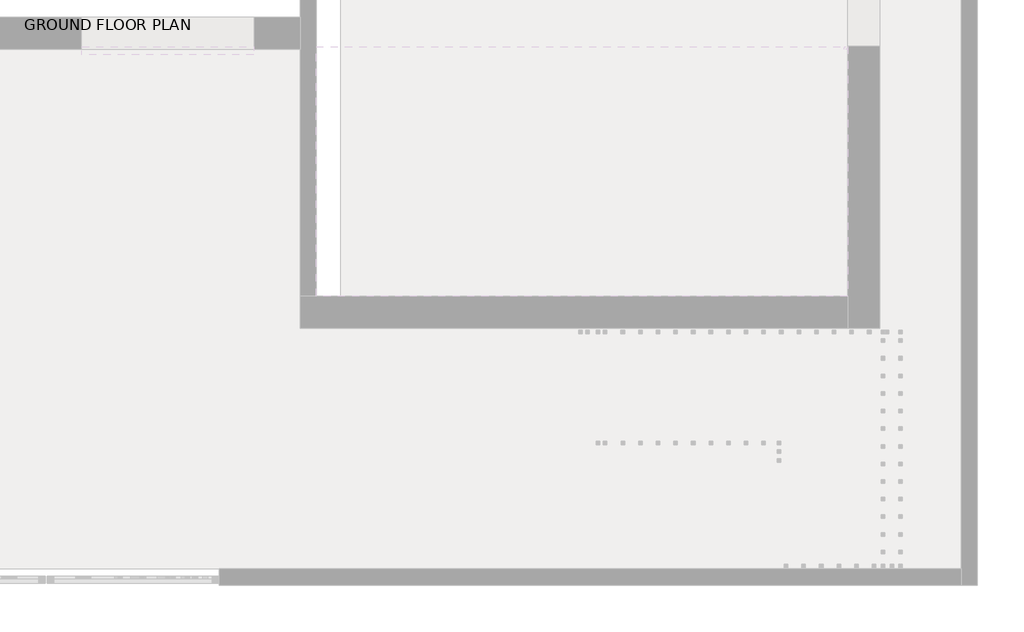
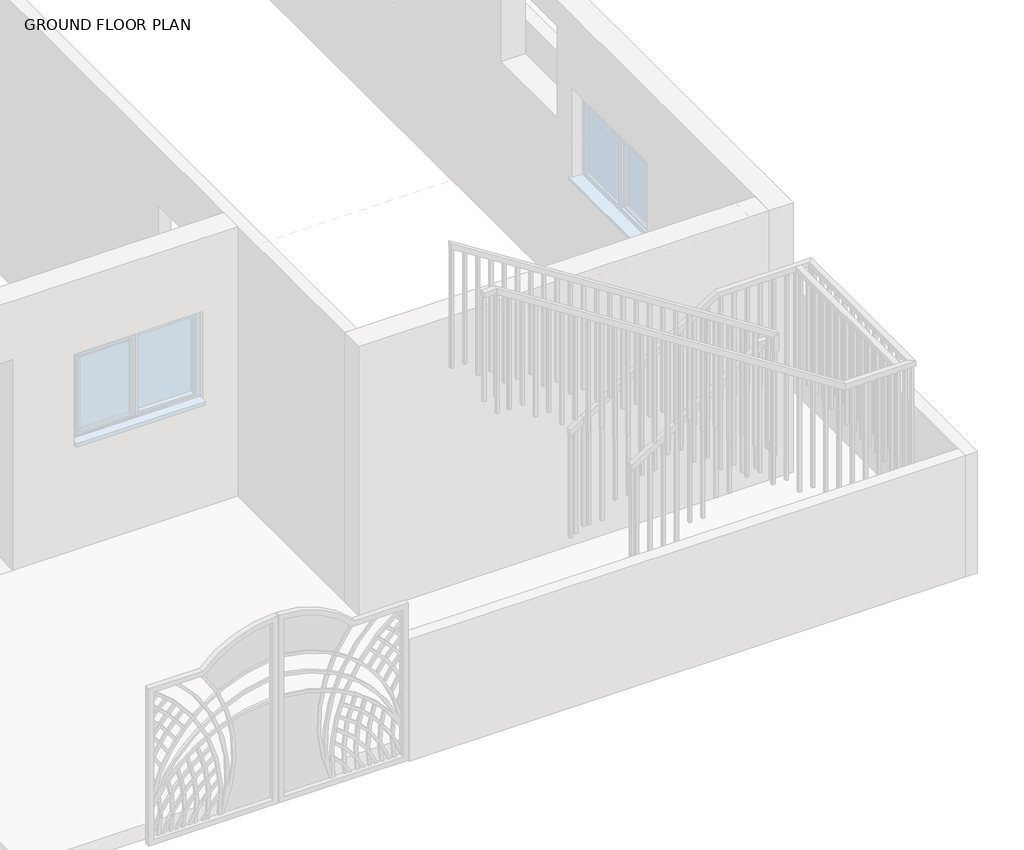
# One storey, part 22 of 23: 2 railings.
"""IFC4 building model written with IfcOpenShell, lengths in millimetres."""

from ifc_helpers import new_model, si_unit, frame, origin, place, context, project, spatial, polyline, outline, extrude, faceted_brep, element, save

model = new_model("IFC4")

# Units and contexts
model_context = context("Model", 3, world=origin())
ifc_project = project(units=[si_unit("LENGTHUNIT", "METRE", prefix="MILLI")], contexts=[model_context])

# Site, building, storey
site = spatial("IfcSite", under=ifc_project)
building = spatial("IfcBuilding", under=site)
storey = spatial("IfcBuildingStorey", under=building, Name="GROUND FLOOR PLAN", Elevation=487.68)

# Railings
placement = place(None, origin())
element("IfcRailing", 1, ObjectType="1100mm", at=placement, inside=storey, context=model_context, shape_type="SolidModel", body=[
    faceted_brep([(-8680.149573, -10220.0521308, 1912.8), (-8680.149573, -10220.0521308, 1853.4423995), (-8680.149573, -10270.0521308, 1853.4423995), (-8680.149573, -10270.0521308, 1912.8), (-7409.7306254, -10220.0521308, 2725.6), (-7395.1045513, -10220.0521308, 2675.6), (-7395.1045513, -10270.0521308, 2675.6), (-7409.7306254, -10270.0521308, 2725.6), (-6495.8132565, -10220.0521308, 2725.6), (-6495.8132565, -10220.0521308, 2675.6), (-6545.8132565, -10270.0521308, 2675.6), (-6545.8132565, -10270.0521308, 2725.6), (-6495.8132565, -11933.6860066, 2725.6), (-6495.8132565, -11933.6860066, 2675.6), (-6545.8132565, -11883.6860066, 2675.6), (-6545.8132565, -11883.6860066, 2725.6), (-7155.718398, -11933.6860066, 2725.6), (-7170.3479429, -11933.6860066, 2675.6), (-7170.3479429, -11883.6860066, 2675.6), (-7155.718398, -11883.6860066, 2725.6), (-10457.8773536, -11933.6860066, 4838.88), (-10457.8773536, -11883.6860066, 4838.88), (-10457.8773536, -11883.6860066, 4779.517542), (-10457.8773536, -11933.6860066, 4779.517542)], [[[0, 1, 2, 3]], [[1, 0, 4, 5]], [[2, 1, 5, 6]], [[3, 2, 6, 7]], [[0, 3, 7, 4]], [[5, 4, 8, 9]], [[6, 5, 9, 10]], [[7, 6, 10, 11]], [[4, 7, 11, 8]], [[9, 8, 12, 13]], [[10, 9, 13, 14]], [[11, 10, 14, 15]], [[8, 11, 15, 12]], [[13, 12, 16, 17]], [[14, 13, 17, 18]], [[15, 14, 18, 19]], [[12, 15, 19, 16]], [[20, 21, 22, 23]], [[17, 16, 20, 23]], [[18, 17, 23, 22]], [[19, 18, 22, 21]], [[16, 19, 21, 20]]]),
    extrude(outline(polyline([(4691.8007425, -10320.8132565), (4707.7999723, -10345.8132565), (3576.32, -10345.8132565), (3576.32, -10320.8132565), (4691.8007425, -10320.8132565)])), frame((0.0, -11921.1860066, 0.0), z_axis=(0.0, 1.0, 0.0), x_axis=(0.0, 0.0, 1.0)), (0.0, 0.0, 1.0), 25.0),
    extrude(outline(polyline([(4611.8045935, -10195.8132565), (4627.8038233, -10220.8132565), (3576.32, -10220.8132565), (3576.32, -10195.8132565), (4611.8045935, -10195.8132565)])), frame((0.0, -11921.1860066, 0.0), z_axis=(0.0, 1.0, 0.0), x_axis=(0.0, 0.0, 1.0)), (0.0, 0.0, 1.0), 25.0),
    extrude(outline(polyline([(4531.8084444, -10070.8132565), (4547.8076742, -10095.8132565), (3413.76, -10095.8132565), (3413.76, -10070.8132565), (4531.8084444, -10070.8132565)])), frame((0.0, -11921.1860066, 0.0), z_axis=(0.0, 1.0, 0.0), x_axis=(0.0, 0.0, 1.0)), (0.0, 0.0, 1.0), 25.0),
    extrude(outline(polyline([(4451.8122954, -9945.8132565), (4467.8115252, -9970.8132565), (3413.76, -9970.8132565), (3413.76, -9945.8132565), (4451.8122954, -9945.8132565)])), frame((0.0, -11921.1860066, 0.0), z_axis=(0.0, 1.0, 0.0), x_axis=(0.0, 0.0, 1.0)), (0.0, 0.0, 1.0), 25.0),
    extrude(outline(polyline([(4371.8161463, -9820.8132565), (4387.8153761, -9845.8132565), (3251.2, -9845.8132565), (3251.2, -9820.8132565), (4371.8161463, -9820.8132565)])), frame((0.0, -11921.1860066, 0.0), z_axis=(0.0, 1.0, 0.0), x_axis=(0.0, 0.0, 1.0)), (0.0, 0.0, 1.0), 25.0),
    extrude(outline(polyline([(4291.8423995, -9695.8132565), (4307.8371231, -9720.8132565), (3251.2, -9720.8132565), (3251.2, -9695.8132565), (4291.8423995, -9695.8132565)])), frame((0.0, -11921.1860066, 0.0), z_axis=(0.0, 1.0, 0.0), x_axis=(0.0, 0.0, 1.0)), (0.0, 0.0, 1.0), 25.0),
    extrude(outline(polyline([(4211.8238482, -9570.8132565), (4227.823078, -9595.8132565), (3088.64, -9595.8132565), (3088.64, -9570.8132565), (4211.8238482, -9570.8132565)])), frame((0.0, -11921.1860066, 0.0), z_axis=(0.0, 1.0, 0.0), x_axis=(0.0, 0.0, 1.0)), (0.0, 0.0, 1.0), 25.0),
    extrude(outline(polyline([(4131.8276992, -9445.8132565), (4147.826929, -9470.8132565), (3088.64, -9470.8132565), (3088.64, -9445.8132565), (4131.8276992, -9445.8132565)])), frame((0.0, -11921.1860066, 0.0), z_axis=(0.0, 1.0, 0.0), x_axis=(0.0, 0.0, 1.0)), (0.0, 0.0, 1.0), 25.0),
    extrude(outline(polyline([(4051.8315501, -9320.8132565), (4067.8307799, -9345.8132565), (2926.08, -9345.8132565), (2926.08, -9320.8132565), (4051.8315501, -9320.8132565)])), frame((0.0, -11921.1860066, 0.0), z_axis=(0.0, 1.0, 0.0), x_axis=(0.0, 0.0, 1.0)), (0.0, 0.0, 1.0), 25.0),
    extrude(outline(polyline([(3971.835401, -9195.8132565), (3987.8346309, -9220.8132565), (2926.08, -9220.8132565), (2926.08, -9195.8132565), (3971.835401, -9195.8132565)])), frame((0.0, -11921.1860066, 0.0), z_axis=(0.0, 1.0, 0.0), x_axis=(0.0, 0.0, 1.0)), (0.0, 0.0, 1.0), 25.0),
    extrude(outline(polyline([(3891.839252, -9070.8132565), (3907.8384818, -9095.8132565), (2763.52, -9095.8132565), (2763.52, -9070.8132565), (3891.839252, -9070.8132565)])), frame((0.0, -11921.1860066, 0.0), z_axis=(0.0, 1.0, 0.0), x_axis=(0.0, 0.0, 1.0)), (0.0, 0.0, 1.0), 25.0),
    extrude(outline(polyline([(3811.8431029, -8945.8132565), (3827.8423328, -8970.8132565), (2763.52, -8970.8132565), (2763.52, -8945.8132565), (3811.8431029, -8945.8132565)])), frame((0.0, -11921.1860066, 0.0), z_axis=(0.0, 1.0, 0.0), x_axis=(0.0, 0.0, 1.0)), (0.0, 0.0, 1.0), 25.0),
    extrude(outline(polyline([(3731.8469539, -8820.8132565), (3747.8461837, -8845.8132565), (2600.96, -8845.8132565), (2600.96, -8820.8132565), (3731.8469539, -8820.8132565)])), frame((0.0, -11921.1860066, 0.0), z_axis=(0.0, 1.0, 0.0), x_axis=(0.0, 0.0, 1.0)), (0.0, 0.0, 1.0), 25.0),
    extrude(outline(polyline([(3651.8508048, -8695.8132565), (3667.8500347, -8720.8132565), (2600.96, -8720.8132565), (2600.96, -8695.8132565), (3651.8508048, -8695.8132565)])), frame((0.0, -11921.1860066, 0.0), z_axis=(0.0, 1.0, 0.0), x_axis=(0.0, 0.0, 1.0)), (0.0, 0.0, 1.0), 25.0),
    extrude(outline(polyline([(3571.8546558, -8570.8132565), (3587.8538856, -8595.8132565), (2438.4, -8595.8132565), (2438.4, -8570.8132565), (3571.8546558, -8570.8132565)])), frame((0.0, -11921.1860066, 0.0), z_axis=(0.0, 1.0, 0.0), x_axis=(0.0, 0.0, 1.0)), (0.0, 0.0, 1.0), 25.0),
    extrude(outline(polyline([(3491.8585067, -8445.8132565), (3507.8577365, -8470.8132565), (2438.4, -8470.8132565), (2438.4, -8445.8132565), (3491.8585067, -8445.8132565)])), frame((0.0, -11921.1860066, 0.0), z_axis=(0.0, 1.0, 0.0), x_axis=(0.0, 0.0, 1.0)), (0.0, 0.0, 1.0), 25.0),
    extrude(outline(polyline([(3411.8623577, -8320.8132565), (3427.8615875, -8345.8132565), (2275.84, -8345.8132565), (2275.84, -8320.8132565), (3411.8623577, -8320.8132565)])), frame((0.0, -11921.1860066, 0.0), z_axis=(0.0, 1.0, 0.0), x_axis=(0.0, 0.0, 1.0)), (0.0, 0.0, 1.0), 25.0),
    extrude(outline(polyline([(3331.8662086, -8195.8132565), (3347.8654384, -8220.8132565), (2275.84, -8220.8132565), (2275.84, -8195.8132565), (3331.8662086, -8195.8132565)])), frame((0.0, -11921.1860066, 0.0), z_axis=(0.0, 1.0, 0.0), x_axis=(0.0, 0.0, 1.0)), (0.0, 0.0, 1.0), 25.0),
    extrude(outline(polyline([(3251.8700596, -8070.8132565), (3267.8692894, -8095.8132565), (2113.28, -8095.8132565), (2113.28, -8070.8132565), (3251.8700596, -8070.8132565)])), frame((0.0, -11921.1860066, 0.0), z_axis=(0.0, 1.0, 0.0), x_axis=(0.0, 0.0, 1.0)), (0.0, 0.0, 1.0), 25.0),
    extrude(outline(polyline([(3171.8739105, -7945.8132565), (3187.8731403, -7970.8132565), (2113.28, -7970.8132565), (2113.28, -7945.8132565), (3171.8739105, -7945.8132565)])), frame((0.0, -11921.1860066, 0.0), z_axis=(0.0, 1.0, 0.0), x_axis=(0.0, 0.0, 1.0)), (0.0, 0.0, 1.0), 25.0),
    extrude(outline(polyline([(3091.8777615, -7820.8132565), (3107.8769913, -7845.8132565), (1950.72, -7845.8132565), (1950.72, -7820.8132565), (3091.8777615, -7820.8132565)])), frame((0.0, -11921.1860066, 0.0), z_axis=(0.0, 1.0, 0.0), x_axis=(0.0, 0.0, 1.0)), (0.0, 0.0, 1.0), 25.0),
    extrude(outline(polyline([(3011.8816124, -7695.8132565), (3027.8808422, -7720.8132565), (1950.72, -7720.8132565), (1950.72, -7695.8132565), (3011.8816124, -7695.8132565)])), frame((0.0, -11921.1860066, 0.0), z_axis=(0.0, 1.0, 0.0), x_axis=(0.0, 0.0, 1.0)), (0.0, 0.0, 1.0), 25.0),
    extrude(outline(polyline([(2931.8854634, -7570.8132565), (2947.8846932, -7595.8132565), (1788.16, -7595.8132565), (1788.16, -7570.8132565), (2931.8854634, -7570.8132565)])), frame((0.0, -11921.1860066, 0.0), z_axis=(0.0, 1.0, 0.0), x_axis=(0.0, 0.0, 1.0)), (0.0, 0.0, 1.0), 25.0),
    extrude(outline(polyline([(2851.8893143, -7445.8132565), (2867.8885441, -7470.8132565), (1788.16, -7470.8132565), (1788.16, -7445.8132565), (2851.8893143, -7445.8132565)])), frame((0.0, -11921.1860066, 0.0), z_axis=(0.0, 1.0, 0.0), x_axis=(0.0, 0.0, 1.0)), (0.0, 0.0, 1.0), 25.0),
    extrude(outline(polyline([(2771.8931653, -7320.8132565), (2787.8923951, -7345.8132565), (1625.6, -7345.8132565), (1625.6, -7320.8132565), (2771.8931653, -7320.8132565)])), frame((0.0, -11921.1860066, 0.0), z_axis=(0.0, 1.0, 0.0), x_axis=(0.0, 0.0, 1.0)), (0.0, 0.0, 1.0), 25.0),
    extrude(outline(polyline([(2691.8970162, -7195.8132565), (2707.896246, -7220.8132565), (1625.6, -7220.8132565), (1625.6, -7195.8132565), (2691.8970162, -7195.8132565)])), frame((0.0, -11921.1860066, 0.0), z_axis=(0.0, 1.0, 0.0), x_axis=(0.0, 0.0, 1.0)), (0.0, 0.0, 1.0), 25.0),
    extrude(outline(polyline([(-7070.8132565, -11921.1860066), (-7095.8132565, -11921.1860066), (-7095.8132565, -11896.1860066), (-7070.8132565, -11896.1860066), (-7070.8132565, -11921.1860066)])), frame((0.0, 0.0, 1625.6), z_axis=(0.0, 0.0, 1.0), x_axis=(1.0, 0.0, 0.0)), (0.0, 0.0, 1.0), 1050.0),
    extrude(outline(polyline([(-6945.8132565, -11921.1860066), (-6970.8132565, -11921.1860066), (-6970.8132565, -11896.1860066), (-6945.8132565, -11896.1860066), (-6945.8132565, -11921.1860066)])), frame((0.0, 0.0, 1625.6), z_axis=(0.0, 0.0, 1.0), x_axis=(1.0, 0.0, 0.0)), (0.0, 0.0, 1.0), 1050.0),
    extrude(outline(polyline([(-6820.8132565, -11921.1860066), (-6845.8132565, -11921.1860066), (-6845.8132565, -11896.1860066), (-6820.8132565, -11896.1860066), (-6820.8132565, -11921.1860066)])), frame((0.0, 0.0, 1625.6), z_axis=(0.0, 0.0, 1.0), x_axis=(1.0, 0.0, 0.0)), (0.0, 0.0, 1.0), 1050.0),
    extrude(outline(polyline([(-6695.8132565, -11921.1860066), (-6720.8132565, -11921.1860066), (-6720.8132565, -11896.1860066), (-6695.8132565, -11896.1860066), (-6695.8132565, -11921.1860066)])), frame((0.0, 0.0, 1625.6), z_axis=(0.0, 0.0, 1.0), x_axis=(1.0, 0.0, 0.0)), (0.0, 0.0, 1.0), 1050.0),
    extrude(outline(polyline([(-6570.8132565, -11921.1860066), (-6595.8132565, -11921.1860066), (-6595.8132565, -11896.1860066), (-6570.8132565, -11896.1860066), (-6570.8132565, -11921.1860066)])), frame((0.0, 0.0, 1625.6), z_axis=(0.0, 0.0, 1.0), x_axis=(1.0, 0.0, 0.0)), (0.0, 0.0, 1.0), 1050.0),
    extrude(outline(polyline([(-6508.3132565, -11795.0521308), (-6508.3132565, -11820.0521308), (-6533.3132565, -11820.0521308), (-6533.3132565, -11795.0521308), (-6508.3132565, -11795.0521308)])), frame((0.0, 0.0, 1625.6), z_axis=(0.0, 0.0, 1.0), x_axis=(1.0, 0.0, 0.0)), (0.0, 0.0, 1.0), 1050.0),
    extrude(outline(polyline([(-6508.3132565, -11670.0521308), (-6508.3132565, -11695.0521308), (-6533.3132565, -11695.0521308), (-6533.3132565, -11670.0521308), (-6508.3132565, -11670.0521308)])), frame((0.0, 0.0, 1625.6), z_axis=(0.0, 0.0, 1.0), x_axis=(1.0, 0.0, 0.0)), (0.0, 0.0, 1.0), 1050.0),
    extrude(outline(polyline([(-6508.3132565, -11545.0521308), (-6508.3132565, -11570.0521308), (-6533.3132565, -11570.0521308), (-6533.3132565, -11545.0521308), (-6508.3132565, -11545.0521308)])), frame((0.0, 0.0, 1625.6), z_axis=(0.0, 0.0, 1.0), x_axis=(1.0, 0.0, 0.0)), (0.0, 0.0, 1.0), 1050.0),
    extrude(outline(polyline([(-6508.3132565, -11420.0521308), (-6508.3132565, -11445.0521308), (-6533.3132565, -11445.0521308), (-6533.3132565, -11420.0521308), (-6508.3132565, -11420.0521308)])), frame((0.0, 0.0, 1625.6), z_axis=(0.0, 0.0, 1.0), x_axis=(1.0, 0.0, 0.0)), (0.0, 0.0, 1.0), 1050.0),
    extrude(outline(polyline([(-6508.3132565, -11295.0521308), (-6508.3132565, -11320.0521308), (-6533.3132565, -11320.0521308), (-6533.3132565, -11295.0521308), (-6508.3132565, -11295.0521308)])), frame((0.0, 0.0, 1625.6), z_axis=(0.0, 0.0, 1.0), x_axis=(1.0, 0.0, 0.0)), (0.0, 0.0, 1.0), 1050.0),
    extrude(outline(polyline([(-6508.3132565, -11170.0521308), (-6508.3132565, -11195.0521308), (-6533.3132565, -11195.0521308), (-6533.3132565, -11170.0521308), (-6508.3132565, -11170.0521308)])), frame((0.0, 0.0, 1625.6), z_axis=(0.0, 0.0, 1.0), x_axis=(1.0, 0.0, 0.0)), (0.0, 0.0, 1.0), 1050.0),
    extrude(outline(polyline([(-6508.3132565, -11045.0521308), (-6508.3132565, -11070.0521308), (-6533.3132565, -11070.0521308), (-6533.3132565, -11045.0521308), (-6508.3132565, -11045.0521308)])), frame((0.0, 0.0, 1625.6), z_axis=(0.0, 0.0, 1.0), x_axis=(1.0, 0.0, 0.0)), (0.0, 0.0, 1.0), 1050.0),
    extrude(outline(polyline([(-6508.3132565, -10920.0521308), (-6508.3132565, -10945.0521308), (-6533.3132565, -10945.0521308), (-6533.3132565, -10920.0521308), (-6508.3132565, -10920.0521308)])), frame((0.0, 0.0, 1625.6), z_axis=(0.0, 0.0, 1.0), x_axis=(1.0, 0.0, 0.0)), (0.0, 0.0, 1.0), 1050.0),
    extrude(outline(polyline([(-6508.3132565, -10795.0521308), (-6508.3132565, -10820.0521308), (-6533.3132565, -10820.0521308), (-6533.3132565, -10795.0521308), (-6508.3132565, -10795.0521308)])), frame((0.0, 0.0, 1625.6), z_axis=(0.0, 0.0, 1.0), x_axis=(1.0, 0.0, 0.0)), (0.0, 0.0, 1.0), 1050.0),
    extrude(outline(polyline([(-6508.3132565, -10670.0521308), (-6508.3132565, -10695.0521308), (-6533.3132565, -10695.0521308), (-6533.3132565, -10670.0521308), (-6508.3132565, -10670.0521308)])), frame((0.0, 0.0, 1625.6), z_axis=(0.0, 0.0, 1.0), x_axis=(1.0, 0.0, 0.0)), (0.0, 0.0, 1.0), 1050.0),
    extrude(outline(polyline([(-6508.3132565, -10545.0521308), (-6508.3132565, -10570.0521308), (-6533.3132565, -10570.0521308), (-6533.3132565, -10545.0521308), (-6508.3132565, -10545.0521308)])), frame((0.0, 0.0, 1625.6), z_axis=(0.0, 0.0, 1.0), x_axis=(1.0, 0.0, 0.0)), (0.0, 0.0, 1.0), 1050.0),
    extrude(outline(polyline([(-6508.3132565, -10420.0521308), (-6508.3132565, -10445.0521308), (-6533.3132565, -10445.0521308), (-6533.3132565, -10420.0521308), (-6508.3132565, -10420.0521308)])), frame((0.0, 0.0, 1625.6), z_axis=(0.0, 0.0, 1.0), x_axis=(1.0, 0.0, 0.0)), (0.0, 0.0, 1.0), 1050.0),
    extrude(outline(polyline([(-6508.3132565, -10295.0521308), (-6508.3132565, -10320.0521308), (-6533.3132565, -10320.0521308), (-6533.3132565, -10295.0521308), (-6508.3132565, -10295.0521308)])), frame((0.0, 0.0, 1625.6), z_axis=(0.0, 0.0, 1.0), x_axis=(1.0, 0.0, 0.0)), (0.0, 0.0, 1.0), 1050.0),
    extrude(outline(polyline([(-6630.149573, -10232.5521308), (-6605.149573, -10232.5521308), (-6605.149573, -10257.5521308), (-6630.149573, -10257.5521308), (-6630.149573, -10232.5521308)])), frame((0.0, 0.0, 1625.6), z_axis=(0.0, 0.0, 1.0), x_axis=(1.0, 0.0, 0.0)), (0.0, 0.0, 1.0), 1050.0),
    extrude(outline(polyline([(-6755.149573, -10232.5521308), (-6730.149573, -10232.5521308), (-6730.149573, -10257.5521308), (-6755.149573, -10257.5521308), (-6755.149573, -10232.5521308)])), frame((0.0, 0.0, 1625.6), z_axis=(0.0, 0.0, 1.0), x_axis=(1.0, 0.0, 0.0)), (0.0, 0.0, 1.0), 1050.0),
    extrude(outline(polyline([(-6880.149573, -10232.5521308), (-6855.149573, -10232.5521308), (-6855.149573, -10257.5521308), (-6880.149573, -10257.5521308), (-6880.149573, -10232.5521308)])), frame((0.0, 0.0, 1625.6), z_axis=(0.0, 0.0, 1.0), x_axis=(1.0, 0.0, 0.0)), (0.0, 0.0, 1.0), 1050.0),
    extrude(outline(polyline([(-7005.149573, -10232.5521308), (-6980.149573, -10232.5521308), (-6980.149573, -10257.5521308), (-7005.149573, -10257.5521308), (-7005.149573, -10232.5521308)])), frame((0.0, 0.0, 1625.6), z_axis=(0.0, 0.0, 1.0), x_axis=(1.0, 0.0, 0.0)), (0.0, 0.0, 1.0), 1050.0),
    extrude(outline(polyline([(-7130.149573, -10232.5521308), (-7105.149573, -10232.5521308), (-7105.149573, -10257.5521308), (-7130.149573, -10257.5521308), (-7130.149573, -10232.5521308)])), frame((0.0, 0.0, 1625.6), z_axis=(0.0, 0.0, 1.0), x_axis=(1.0, 0.0, 0.0)), (0.0, 0.0, 1.0), 1050.0),
    extrude(outline(polyline([(-7255.149573, -10232.5521308), (-7230.149573, -10232.5521308), (-7230.149573, -10257.5521308), (-7255.149573, -10257.5521308), (-7255.149573, -10232.5521308)])), frame((0.0, 0.0, 1625.6), z_axis=(0.0, 0.0, 1.0), x_axis=(1.0, 0.0, 0.0)), (0.0, 0.0, 1.0), 1050.0),
    extrude(outline(polyline([(-7380.149573, -10232.5521308), (-7355.149573, -10232.5521308), (-7355.149573, -10257.5521308), (-7380.149573, -10257.5521308), (-7380.149573, -10232.5521308)])), frame((0.0, 0.0, 1625.6), z_axis=(0.0, 0.0, 1.0), x_axis=(1.0, 0.0, 0.0)), (0.0, 0.0, 1.0), 1050.0),
    extrude(outline(polyline([(1463.04, -7505.149573), (1463.04, -7480.149573), (2621.1891352, -7480.149573), (2605.1944115, -7505.149573), (1463.04, -7505.149573)])), frame((0.0, -10257.5521308, 0.0), z_axis=(0.0, 1.0, 0.0), x_axis=(0.0, 0.0, 1.0)), (0.0, 0.0, 1.0), 25.0),
    extrude(outline(polyline([(1463.04, -7630.149573), (1463.04, -7605.149573), (2541.2155169, -7605.149573), (2525.2207932, -7630.149573), (1463.04, -7630.149573)])), frame((0.0, -10257.5521308, 0.0), z_axis=(0.0, 1.0, 0.0), x_axis=(0.0, 0.0, 1.0)), (0.0, 0.0, 1.0), 25.0),
    extrude(outline(polyline([(1300.48, -7755.149573), (1300.48, -7730.149573), (2461.2418986, -7730.149573), (2445.2471749, -7755.149573), (1300.48, -7755.149573)])), frame((0.0, -10257.5521308, 0.0), z_axis=(0.0, 1.0, 0.0), x_axis=(0.0, 0.0, 1.0)), (0.0, 0.0, 1.0), 25.0),
    extrude(outline(polyline([(1300.48, -7880.149573), (1300.48, -7855.149573), (2381.2682803, -7855.149573), (2365.2735566, -7880.149573), (1300.48, -7880.149573)])), frame((0.0, -10257.5521308, 0.0), z_axis=(0.0, 1.0, 0.0), x_axis=(0.0, 0.0, 1.0)), (0.0, 0.0, 1.0), 25.0),
    extrude(outline(polyline([(1137.92, -8005.149573), (1137.92, -7980.149573), (2301.294662, -7980.149573), (2285.2999383, -8005.149573), (1137.92, -8005.149573)])), frame((0.0, -10257.5521308, 0.0), z_axis=(0.0, 1.0, 0.0), x_axis=(0.0, 0.0, 1.0)), (0.0, 0.0, 1.0), 25.0),
    extrude(outline(polyline([(1137.92, -8130.149573), (1137.92, -8105.149573), (2221.3210437, -8105.149573), (2205.32632, -8130.149573), (1137.92, -8130.149573)])), frame((0.0, -10257.5521308, 0.0), z_axis=(0.0, 1.0, 0.0), x_axis=(0.0, 0.0, 1.0)), (0.0, 0.0, 1.0), 25.0),
    extrude(outline(polyline([(975.36, -8255.149573), (975.36, -8230.149573), (2141.3474254, -8230.149573), (2125.3527017, -8255.149573), (975.36, -8255.149573)])), frame((0.0, -10257.5521308, 0.0), z_axis=(0.0, 1.0, 0.0), x_axis=(0.0, 0.0, 1.0)), (0.0, 0.0, 1.0), 25.0),
    extrude(outline(polyline([(975.36, -8380.149573), (975.36, -8355.149573), (2061.3738071, -8355.149573), (2045.3790834, -8380.149573), (975.36, -8380.149573)])), frame((0.0, -10257.5521308, 0.0), z_axis=(0.0, 1.0, 0.0), x_axis=(0.0, 0.0, 1.0)), (0.0, 0.0, 1.0), 25.0),
    extrude(outline(polyline([(812.8, -8505.149573), (812.8, -8480.149573), (1981.4001888, -8480.149573), (1965.4054651, -8505.149573), (812.8, -8505.149573)])), frame((0.0, -10257.5521308, 0.0), z_axis=(0.0, 1.0, 0.0), x_axis=(0.0, 0.0, 1.0)), (0.0, 0.0, 1.0), 25.0),
    extrude(outline(polyline([(812.8, -8630.149573), (812.8, -8605.149573), (1901.4265705, -8605.149573), (1885.4318468, -8630.149573), (812.8, -8630.149573)])), frame((0.0, -10257.5521308, 0.0), z_axis=(0.0, 1.0, 0.0), x_axis=(0.0, 0.0, 1.0)), (0.0, 0.0, 1.0), 25.0),
    extrude(outline(polyline([(-6508.3132565, -11896.1860066), (-6508.3132565, -11921.1860066), (-6533.3132565, -11921.1860066), (-6533.3132565, -11896.1860066), (-6508.3132565, -11896.1860066)])), frame((0.0, 0.0, 1625.6), z_axis=(0.0, 0.0, 1.0), x_axis=(1.0, 0.0, 0.0)), (0.0, 0.0, 1.0), 1050.0),
    extrude(outline(polyline([(-6533.3132565, -10232.5521308), (-6508.3132565, -10232.5521308), (-6508.3132565, -10257.5521308), (-6533.3132565, -10257.5521308), (-6533.3132565, -10232.5521308)])), frame((0.0, 0.0, 1625.6), z_axis=(0.0, 0.0, 1.0), x_axis=(1.0, 0.0, 0.0)), (0.0, 0.0, 1.0), 1050.0),
    extrude(outline(polyline([(4763.5183122, -10432.8773536), (4779.517542, -10457.8773536), (3576.32, -10457.8773536), (3576.32, -10432.8773536), (4763.5183122, -10432.8773536)])), frame((0.0, -11921.1860066, 0.0), z_axis=(0.0, 1.0, 0.0), x_axis=(0.0, 0.0, 1.0)), (0.0, 0.0, 1.0), 25.0),
    extrude(outline(polyline([(812.8, -8680.149573), (812.8, -8655.149573), (1869.4371231, -8655.149573), (1853.4423995, -8680.149573), (812.8, -8680.149573)])), frame((0.0, -10257.5521308, 0.0), z_axis=(0.0, 1.0, 0.0), x_axis=(0.0, 0.0, 1.0)), (0.0, 0.0, 1.0), 25.0),
])
element("IfcRailing", 2, ObjectType="1100mm", at=placement, inside=storey, context=model_context, shape_type="SolidModel", body=[
    faceted_brep([(-8805.870786, -10220.0521308, 1832.3649576), (-8805.870786, -10220.0521308, 1773.007357), (-8805.870786, -10270.0521308, 1773.007357), (-8805.870786, -10270.0521308, 1832.3649576), (-7409.7306254, -10220.0521308, 2725.6), (-7395.1045513, -10220.0521308, 2675.6), (-7395.1045513, -10270.0521308, 2675.6), (-7409.7306254, -10270.0521308, 2725.6), (-6621.5344696, -10220.0521308, 2725.6), (-6621.5344696, -10220.0521308, 2675.6), (-6671.5344696, -10270.0521308, 2675.6), (-6671.5344696, -10270.0521308, 2725.6), (-6621.5344696, -11933.6860066, 2725.6), (-6621.5344696, -11933.6860066, 2675.6), (-6671.5344696, -11883.6860066, 2675.6), (-6671.5344696, -11883.6860066, 2725.6), (-7155.718398, -11933.6860066, 2725.6), (-7170.3479429, -11933.6860066, 2675.6), (-7170.3479429, -11883.6860066, 2675.6), (-7155.718398, -11883.6860066, 2725.6), (-10457.8773536, -11933.6860066, 4838.88), (-10472.5068984, -11933.6860066, 4788.88), (-10472.5068984, -11883.6860066, 4788.88), (-10457.8773536, -11883.6860066, 4838.88), (-10583.5985666, -11933.6860066, 4838.88), (-10583.5985666, -11883.6860066, 4838.88), (-10583.5985666, -11883.6860066, 4788.88), (-10583.5985666, -11933.6860066, 4788.88)], [[[0, 1, 2, 3]], [[1, 0, 4, 5]], [[2, 1, 5, 6]], [[3, 2, 6, 7]], [[0, 3, 7, 4]], [[5, 4, 8, 9]], [[6, 5, 9, 10]], [[7, 6, 10, 11]], [[4, 7, 11, 8]], [[9, 8, 12, 13]], [[10, 9, 13, 14]], [[11, 10, 14, 15]], [[8, 11, 15, 12]], [[13, 12, 16, 17]], [[14, 13, 17, 18]], [[15, 14, 18, 19]], [[12, 15, 19, 16]], [[17, 16, 20, 21]], [[18, 17, 21, 22]], [[19, 18, 22, 23]], [[16, 19, 23, 20]], [[24, 25, 26, 27]], [[21, 20, 24, 27]], [[22, 21, 27, 26]], [[23, 22, 26, 25]], [[20, 23, 25, 24]]]),
    extrude(outline(polyline([(-10446.5344696, -11921.1860066), (-10471.5344696, -11921.1860066), (-10471.5344696, -11896.1860066), (-10446.5344696, -11896.1860066), (-10446.5344696, -11921.1860066)])), frame((0.0, 0.0, 3738.88), z_axis=(0.0, 0.0, 1.0), x_axis=(1.0, 0.0, 0.0)), (0.0, 0.0, 1.0), 1050.0),
    extrude(outline(polyline([(4692.2622966, -10321.5344696), (4708.2615264, -10346.5344696), (3576.32, -10346.5344696), (3576.32, -10321.5344696), (4692.2622966, -10321.5344696)])), frame((0.0, -11921.1860066, 0.0), z_axis=(0.0, 1.0, 0.0), x_axis=(0.0, 0.0, 1.0)), (0.0, 0.0, 1.0), 25.0),
    extrude(outline(polyline([(4612.2661476, -10196.5344696), (4628.2653774, -10221.5344696), (3576.32, -10221.5344696), (3576.32, -10196.5344696), (4612.2661476, -10196.5344696)])), frame((0.0, -11921.1860066, 0.0), z_axis=(0.0, 1.0, 0.0), x_axis=(0.0, 0.0, 1.0)), (0.0, 0.0, 1.0), 25.0),
    extrude(outline(polyline([(4532.2699985, -10071.5344696), (4548.2692283, -10096.5344696), (3413.76, -10096.5344696), (3413.76, -10071.5344696), (4532.2699985, -10071.5344696)])), frame((0.0, -11921.1860066, 0.0), z_axis=(0.0, 1.0, 0.0), x_axis=(0.0, 0.0, 1.0)), (0.0, 0.0, 1.0), 25.0),
    extrude(outline(polyline([(4452.2738495, -9946.5344696), (4468.2730793, -9971.5344696), (3413.76, -9971.5344696), (3413.76, -9946.5344696), (4452.2738495, -9946.5344696)])), frame((0.0, -11921.1860066, 0.0), z_axis=(0.0, 1.0, 0.0), x_axis=(0.0, 0.0, 1.0)), (0.0, 0.0, 1.0), 25.0),
    extrude(outline(polyline([(4372.2777004, -9821.5344696), (4388.2769302, -9846.5344696), (3251.2, -9846.5344696), (3251.2, -9821.5344696), (4372.2777004, -9821.5344696)])), frame((0.0, -11921.1860066, 0.0), z_axis=(0.0, 1.0, 0.0), x_axis=(0.0, 0.0, 1.0)), (0.0, 0.0, 1.0), 25.0),
    extrude(outline(polyline([(4292.2815514, -9696.5344696), (4308.2807812, -9721.5344696), (3251.2, -9721.5344696), (3251.2, -9696.5344696), (4292.2815514, -9696.5344696)])), frame((0.0, -11921.1860066, 0.0), z_axis=(0.0, 1.0, 0.0), x_axis=(0.0, 0.0, 1.0)), (0.0, 0.0, 1.0), 25.0),
    extrude(outline(polyline([(4212.2854023, -9571.5344696), (4228.2846321, -9596.5344696), (3088.64, -9596.5344696), (3088.64, -9571.5344696), (4212.2854023, -9571.5344696)])), frame((0.0, -11921.1860066, 0.0), z_axis=(0.0, 1.0, 0.0), x_axis=(0.0, 0.0, 1.0)), (0.0, 0.0, 1.0), 25.0),
    extrude(outline(polyline([(4132.2892533, -9446.5344696), (4148.2884831, -9471.5344696), (3088.64, -9471.5344696), (3088.64, -9446.5344696), (4132.2892533, -9446.5344696)])), frame((0.0, -11921.1860066, 0.0), z_axis=(0.0, 1.0, 0.0), x_axis=(0.0, 0.0, 1.0)), (0.0, 0.0, 1.0), 25.0),
    extrude(outline(polyline([(4052.2931042, -9321.5344696), (4068.292334, -9346.5344696), (2926.08, -9346.5344696), (2926.08, -9321.5344696), (4052.2931042, -9321.5344696)])), frame((0.0, -11921.1860066, 0.0), z_axis=(0.0, 1.0, 0.0), x_axis=(0.0, 0.0, 1.0)), (0.0, 0.0, 1.0), 25.0),
    extrude(outline(polyline([(3972.2969552, -9196.5344696), (3988.296185, -9221.5344696), (2926.08, -9221.5344696), (2926.08, -9196.5344696), (3972.2969552, -9196.5344696)])), frame((0.0, -11921.1860066, 0.0), z_axis=(0.0, 1.0, 0.0), x_axis=(0.0, 0.0, 1.0)), (0.0, 0.0, 1.0), 25.0),
    extrude(outline(polyline([(3892.3008061, -9071.5344696), (3908.3000359, -9096.5344696), (2763.52, -9096.5344696), (2763.52, -9071.5344696), (3892.3008061, -9071.5344696)])), frame((0.0, -11921.1860066, 0.0), z_axis=(0.0, 1.0, 0.0), x_axis=(0.0, 0.0, 1.0)), (0.0, 0.0, 1.0), 25.0),
    extrude(outline(polyline([(3812.3046571, -8946.5344696), (3828.3038869, -8971.5344696), (2763.52, -8971.5344696), (2763.52, -8946.5344696), (3812.3046571, -8946.5344696)])), frame((0.0, -11921.1860066, 0.0), z_axis=(0.0, 1.0, 0.0), x_axis=(0.0, 0.0, 1.0)), (0.0, 0.0, 1.0), 25.0),
    extrude(outline(polyline([(3732.308508, -8821.5344696), (3748.3077378, -8846.5344696), (2600.96, -8846.5344696), (2600.96, -8821.5344696), (3732.308508, -8821.5344696)])), frame((0.0, -11921.1860066, 0.0), z_axis=(0.0, 1.0, 0.0), x_axis=(0.0, 0.0, 1.0)), (0.0, 0.0, 1.0), 25.0),
    extrude(outline(polyline([(3652.312359, -8696.5344696), (3668.3115888, -8721.5344696), (2600.96, -8721.5344696), (2600.96, -8696.5344696), (3652.312359, -8696.5344696)])), frame((0.0, -11921.1860066, 0.0), z_axis=(0.0, 1.0, 0.0), x_axis=(0.0, 0.0, 1.0)), (0.0, 0.0, 1.0), 25.0),
    extrude(outline(polyline([(3572.3162099, -8571.5344696), (3588.3154397, -8596.5344696), (2438.4, -8596.5344696), (2438.4, -8571.5344696), (3572.3162099, -8571.5344696)])), frame((0.0, -11921.1860066, 0.0), z_axis=(0.0, 1.0, 0.0), x_axis=(0.0, 0.0, 1.0)), (0.0, 0.0, 1.0), 25.0),
    extrude(outline(polyline([(3492.3200609, -8446.5344696), (3508.3192907, -8471.5344696), (2438.4, -8471.5344696), (2438.4, -8446.5344696), (3492.3200609, -8446.5344696)])), frame((0.0, -11921.1860066, 0.0), z_axis=(0.0, 1.0, 0.0), x_axis=(0.0, 0.0, 1.0)), (0.0, 0.0, 1.0), 25.0),
    extrude(outline(polyline([(3412.3239118, -8321.5344696), (3428.3231416, -8346.5344696), (2275.84, -8346.5344696), (2275.84, -8321.5344696), (3412.3239118, -8321.5344696)])), frame((0.0, -11921.1860066, 0.0), z_axis=(0.0, 1.0, 0.0), x_axis=(0.0, 0.0, 1.0)), (0.0, 0.0, 1.0), 25.0),
    extrude(outline(polyline([(3332.3277628, -8196.5344696), (3348.3269926, -8221.5344696), (2275.84, -8221.5344696), (2275.84, -8196.5344696), (3332.3277628, -8196.5344696)])), frame((0.0, -11921.1860066, 0.0), z_axis=(0.0, 1.0, 0.0), x_axis=(0.0, 0.0, 1.0)), (0.0, 0.0, 1.0), 25.0),
    extrude(outline(polyline([(3252.3316137, -8071.5344696), (3268.3308435, -8096.5344696), (2113.28, -8096.5344696), (2113.28, -8071.5344696), (3252.3316137, -8071.5344696)])), frame((0.0, -11921.1860066, 0.0), z_axis=(0.0, 1.0, 0.0), x_axis=(0.0, 0.0, 1.0)), (0.0, 0.0, 1.0), 25.0),
    extrude(outline(polyline([(3172.3354647, -7946.5344696), (3188.3346945, -7971.5344696), (2113.28, -7971.5344696), (2113.28, -7946.5344696), (3172.3354647, -7946.5344696)])), frame((0.0, -11921.1860066, 0.0), z_axis=(0.0, 1.0, 0.0), x_axis=(0.0, 0.0, 1.0)), (0.0, 0.0, 1.0), 25.0),
    extrude(outline(polyline([(3092.4129874, -7821.5344696), (3108.4077111, -7846.5344696), (1950.72, -7846.5344696), (1950.72, -7821.5344696), (3092.4129874, -7821.5344696)])), frame((0.0, -11921.1860066, 0.0), z_axis=(0.0, 1.0, 0.0), x_axis=(0.0, 0.0, 1.0)), (0.0, 0.0, 1.0), 25.0),
    extrude(outline(polyline([(3012.4393691, -7696.5344696), (3028.4340928, -7721.5344696), (1950.72, -7721.5344696), (1950.72, -7696.5344696), (3012.4393691, -7696.5344696)])), frame((0.0, -11921.1860066, 0.0), z_axis=(0.0, 1.0, 0.0), x_axis=(0.0, 0.0, 1.0)), (0.0, 0.0, 1.0), 25.0),
    extrude(outline(polyline([(2932.4657508, -7571.5344696), (2948.4604745, -7596.5344696), (1788.16, -7596.5344696), (1788.16, -7571.5344696), (2932.4657508, -7571.5344696)])), frame((0.0, -11921.1860066, 0.0), z_axis=(0.0, 1.0, 0.0), x_axis=(0.0, 0.0, 1.0)), (0.0, 0.0, 1.0), 25.0),
    extrude(outline(polyline([(2852.4921325, -7446.5344696), (2868.4868562, -7471.5344696), (1788.16, -7471.5344696), (1788.16, -7446.5344696), (2852.4921325, -7446.5344696)])), frame((0.0, -11921.1860066, 0.0), z_axis=(0.0, 1.0, 0.0), x_axis=(0.0, 0.0, 1.0)), (0.0, 0.0, 1.0), 25.0),
    extrude(outline(polyline([(2772.3547194, -7321.5344696), (2788.3539492, -7346.5344696), (1625.6, -7346.5344696), (1625.6, -7321.5344696), (2772.3547194, -7321.5344696)])), frame((0.0, -11921.1860066, 0.0), z_axis=(0.0, 1.0, 0.0), x_axis=(0.0, 0.0, 1.0)), (0.0, 0.0, 1.0), 25.0),
    extrude(outline(polyline([(2692.3585703, -7196.5344696), (2708.3578001, -7221.5344696), (1625.6, -7221.5344696), (1625.6, -7196.5344696), (2692.3585703, -7196.5344696)])), frame((0.0, -11921.1860066, 0.0), z_axis=(0.0, 1.0, 0.0), x_axis=(0.0, 0.0, 1.0)), (0.0, 0.0, 1.0), 25.0),
    extrude(outline(polyline([(-7071.5344696, -11921.1860066), (-7096.5344696, -11921.1860066), (-7096.5344696, -11896.1860066), (-7071.5344696, -11896.1860066), (-7071.5344696, -11921.1860066)])), frame((0.0, 0.0, 1625.6), z_axis=(0.0, 0.0, 1.0), x_axis=(1.0, 0.0, 0.0)), (0.0, 0.0, 1.0), 1050.0),
    extrude(outline(polyline([(-6946.5344696, -11921.1860066), (-6971.5344696, -11921.1860066), (-6971.5344696, -11896.1860066), (-6946.5344696, -11896.1860066), (-6946.5344696, -11921.1860066)])), frame((0.0, 0.0, 1625.6), z_axis=(0.0, 0.0, 1.0), x_axis=(1.0, 0.0, 0.0)), (0.0, 0.0, 1.0), 1050.0),
    extrude(outline(polyline([(-6821.5344696, -11921.1860066), (-6846.5344696, -11921.1860066), (-6846.5344696, -11896.1860066), (-6821.5344696, -11896.1860066), (-6821.5344696, -11921.1860066)])), frame((0.0, 0.0, 1625.6), z_axis=(0.0, 0.0, 1.0), x_axis=(1.0, 0.0, 0.0)), (0.0, 0.0, 1.0), 1050.0),
    extrude(outline(polyline([(-6696.5344696, -11921.1860066), (-6721.5344696, -11921.1860066), (-6721.5344696, -11896.1860066), (-6696.5344696, -11896.1860066), (-6696.5344696, -11921.1860066)])), frame((0.0, 0.0, 1625.6), z_axis=(0.0, 0.0, 1.0), x_axis=(1.0, 0.0, 0.0)), (0.0, 0.0, 1.0), 1050.0),
    extrude(outline(polyline([(-6634.0344696, -11795.0521308), (-6634.0344696, -11820.0521308), (-6659.0344696, -11820.0521308), (-6659.0344696, -11795.0521308), (-6634.0344696, -11795.0521308)])), frame((0.0, 0.0, 1625.6), z_axis=(0.0, 0.0, 1.0), x_axis=(1.0, 0.0, 0.0)), (0.0, 0.0, 1.0), 1050.0),
    extrude(outline(polyline([(-6634.0344696, -11670.0521308), (-6634.0344696, -11695.0521308), (-6659.0344696, -11695.0521308), (-6659.0344696, -11670.0521308), (-6634.0344696, -11670.0521308)])), frame((0.0, 0.0, 1625.6), z_axis=(0.0, 0.0, 1.0), x_axis=(1.0, 0.0, 0.0)), (0.0, 0.0, 1.0), 1050.0),
    extrude(outline(polyline([(-6634.0344696, -11545.0521308), (-6634.0344696, -11570.0521308), (-6659.0344696, -11570.0521308), (-6659.0344696, -11545.0521308), (-6634.0344696, -11545.0521308)])), frame((0.0, 0.0, 1625.6), z_axis=(0.0, 0.0, 1.0), x_axis=(1.0, 0.0, 0.0)), (0.0, 0.0, 1.0), 1050.0),
    extrude(outline(polyline([(-6634.0344696, -11420.0521308), (-6634.0344696, -11445.0521308), (-6659.0344696, -11445.0521308), (-6659.0344696, -11420.0521308), (-6634.0344696, -11420.0521308)])), frame((0.0, 0.0, 1625.6), z_axis=(0.0, 0.0, 1.0), x_axis=(1.0, 0.0, 0.0)), (0.0, 0.0, 1.0), 1050.0),
    extrude(outline(polyline([(-6634.0344696, -11295.0521308), (-6634.0344696, -11320.0521308), (-6659.0344696, -11320.0521308), (-6659.0344696, -11295.0521308), (-6634.0344696, -11295.0521308)])), frame((0.0, 0.0, 1625.6), z_axis=(0.0, 0.0, 1.0), x_axis=(1.0, 0.0, 0.0)), (0.0, 0.0, 1.0), 1050.0),
    extrude(outline(polyline([(-6634.0344696, -11170.0521308), (-6634.0344696, -11195.0521308), (-6659.0344696, -11195.0521308), (-6659.0344696, -11170.0521308), (-6634.0344696, -11170.0521308)])), frame((0.0, 0.0, 1625.6), z_axis=(0.0, 0.0, 1.0), x_axis=(1.0, 0.0, 0.0)), (0.0, 0.0, 1.0), 1050.0),
    extrude(outline(polyline([(-6634.0344696, -11045.0521308), (-6634.0344696, -11070.0521308), (-6659.0344696, -11070.0521308), (-6659.0344696, -11045.0521308), (-6634.0344696, -11045.0521308)])), frame((0.0, 0.0, 1625.6), z_axis=(0.0, 0.0, 1.0), x_axis=(1.0, 0.0, 0.0)), (0.0, 0.0, 1.0), 1050.0),
    extrude(outline(polyline([(-6634.0344696, -10920.0521308), (-6634.0344696, -10945.0521308), (-6659.0344696, -10945.0521308), (-6659.0344696, -10920.0521308), (-6634.0344696, -10920.0521308)])), frame((0.0, 0.0, 1625.6), z_axis=(0.0, 0.0, 1.0), x_axis=(1.0, 0.0, 0.0)), (0.0, 0.0, 1.0), 1050.0),
    extrude(outline(polyline([(-6634.0344696, -10795.0521308), (-6634.0344696, -10820.0521308), (-6659.0344696, -10820.0521308), (-6659.0344696, -10795.0521308), (-6634.0344696, -10795.0521308)])), frame((0.0, 0.0, 1625.6), z_axis=(0.0, 0.0, 1.0), x_axis=(1.0, 0.0, 0.0)), (0.0, 0.0, 1.0), 1050.0),
    extrude(outline(polyline([(-6634.0344696, -10670.0521308), (-6634.0344696, -10695.0521308), (-6659.0344696, -10695.0521308), (-6659.0344696, -10670.0521308), (-6634.0344696, -10670.0521308)])), frame((0.0, 0.0, 1625.6), z_axis=(0.0, 0.0, 1.0), x_axis=(1.0, 0.0, 0.0)), (0.0, 0.0, 1.0), 1050.0),
    extrude(outline(polyline([(-6634.0344696, -10545.0521308), (-6634.0344696, -10570.0521308), (-6659.0344696, -10570.0521308), (-6659.0344696, -10545.0521308), (-6634.0344696, -10545.0521308)])), frame((0.0, 0.0, 1625.6), z_axis=(0.0, 0.0, 1.0), x_axis=(1.0, 0.0, 0.0)), (0.0, 0.0, 1.0), 1050.0),
    extrude(outline(polyline([(-6634.0344696, -10420.0521308), (-6634.0344696, -10445.0521308), (-6659.0344696, -10445.0521308), (-6659.0344696, -10420.0521308), (-6634.0344696, -10420.0521308)])), frame((0.0, 0.0, 1625.6), z_axis=(0.0, 0.0, 1.0), x_axis=(1.0, 0.0, 0.0)), (0.0, 0.0, 1.0), 1050.0),
    extrude(outline(polyline([(-6634.0344696, -10295.0521308), (-6634.0344696, -10320.0521308), (-6659.0344696, -10320.0521308), (-6659.0344696, -10295.0521308), (-6634.0344696, -10295.0521308)])), frame((0.0, 0.0, 1625.6), z_axis=(0.0, 0.0, 1.0), x_axis=(1.0, 0.0, 0.0)), (0.0, 0.0, 1.0), 1050.0),
    extrude(outline(polyline([(-6755.870786, -10232.5521308), (-6730.870786, -10232.5521308), (-6730.870786, -10257.5521308), (-6755.870786, -10257.5521308), (-6755.870786, -10232.5521308)])), frame((0.0, 0.0, 1625.6), z_axis=(0.0, 0.0, 1.0), x_axis=(1.0, 0.0, 0.0)), (0.0, 0.0, 1.0), 1050.0),
    extrude(outline(polyline([(-6880.870786, -10232.5521308), (-6855.870786, -10232.5521308), (-6855.870786, -10257.5521308), (-6880.870786, -10257.5521308), (-6880.870786, -10232.5521308)])), frame((0.0, 0.0, 1625.6), z_axis=(0.0, 0.0, 1.0), x_axis=(1.0, 0.0, 0.0)), (0.0, 0.0, 1.0), 1050.0),
    extrude(outline(polyline([(-7005.870786, -10232.5521308), (-6980.870786, -10232.5521308), (-6980.870786, -10257.5521308), (-7005.870786, -10257.5521308), (-7005.870786, -10232.5521308)])), frame((0.0, 0.0, 1625.6), z_axis=(0.0, 0.0, 1.0), x_axis=(1.0, 0.0, 0.0)), (0.0, 0.0, 1.0), 1050.0),
    extrude(outline(polyline([(-7130.870786, -10232.5521308), (-7105.870786, -10232.5521308), (-7105.870786, -10257.5521308), (-7130.870786, -10257.5521308), (-7130.870786, -10232.5521308)])), frame((0.0, 0.0, 1625.6), z_axis=(0.0, 0.0, 1.0), x_axis=(1.0, 0.0, 0.0)), (0.0, 0.0, 1.0), 1050.0),
    extrude(outline(polyline([(-7255.870786, -10232.5521308), (-7230.870786, -10232.5521308), (-7230.870786, -10257.5521308), (-7255.870786, -10257.5521308), (-7255.870786, -10232.5521308)])), frame((0.0, 0.0, 1625.6), z_axis=(0.0, 0.0, 1.0), x_axis=(1.0, 0.0, 0.0)), (0.0, 0.0, 1.0), 1050.0),
    extrude(outline(polyline([(-7380.870786, -10232.5521308), (-7355.870786, -10232.5521308), (-7355.870786, -10257.5521308), (-7380.870786, -10257.5521308), (-7380.870786, -10232.5521308)])), frame((0.0, 0.0, 1625.6), z_axis=(0.0, 0.0, 1.0), x_axis=(1.0, 0.0, 0.0)), (0.0, 0.0, 1.0), 1050.0),
    extrude(outline(polyline([(1463.04, -7505.870786), (1463.04, -7480.870786), (2620.7277111, -7480.870786), (2604.7329874, -7505.870786), (1463.04, -7505.870786)])), frame((0.0, -10257.5521308, 0.0), z_axis=(0.0, 1.0, 0.0), x_axis=(0.0, 0.0, 1.0)), (0.0, 0.0, 1.0), 25.0),
    extrude(outline(polyline([(1463.04, -7630.870786), (1463.04, -7605.870786), (2540.7540928, -7605.870786), (2524.7593691, -7630.870786), (1463.04, -7630.870786)])), frame((0.0, -10257.5521308, 0.0), z_axis=(0.0, 1.0, 0.0), x_axis=(0.0, 0.0, 1.0)), (0.0, 0.0, 1.0), 25.0),
    extrude(outline(polyline([(1300.48, -7755.870786), (1300.48, -7730.870786), (2460.7804745, -7730.870786), (2444.7857508, -7755.870786), (1300.48, -7755.870786)])), frame((0.0, -10257.5521308, 0.0), z_axis=(0.0, 1.0, 0.0), x_axis=(0.0, 0.0, 1.0)), (0.0, 0.0, 1.0), 25.0),
    extrude(outline(polyline([(1300.48, -7880.870786), (1300.48, -7855.870786), (2380.8068562, -7855.870786), (2364.8121325, -7880.870786), (1300.48, -7880.870786)])), frame((0.0, -10257.5521308, 0.0), z_axis=(0.0, 1.0, 0.0), x_axis=(0.0, 0.0, 1.0)), (0.0, 0.0, 1.0), 25.0),
    extrude(outline(polyline([(1137.92, -8005.870786), (1137.92, -7980.870786), (2300.8332379, -7980.870786), (2284.8385142, -8005.870786), (1137.92, -8005.870786)])), frame((0.0, -10257.5521308, 0.0), z_axis=(0.0, 1.0, 0.0), x_axis=(0.0, 0.0, 1.0)), (0.0, 0.0, 1.0), 25.0),
    extrude(outline(polyline([(1137.92, -8130.870786), (1137.92, -8105.870786), (2220.8596196, -8105.870786), (2204.8648959, -8130.870786), (1137.92, -8130.870786)])), frame((0.0, -10257.5521308, 0.0), z_axis=(0.0, 1.0, 0.0), x_axis=(0.0, 0.0, 1.0)), (0.0, 0.0, 1.0), 25.0),
    extrude(outline(polyline([(975.36, -8255.870786), (975.36, -8230.870786), (2140.8860012, -8230.870786), (2124.8912776, -8255.870786), (975.36, -8255.870786)])), frame((0.0, -10257.5521308, 0.0), z_axis=(0.0, 1.0, 0.0), x_axis=(0.0, 0.0, 1.0)), (0.0, 0.0, 1.0), 25.0),
    extrude(outline(polyline([(975.36, -8380.870786), (975.36, -8355.870786), (2060.9123829, -8355.870786), (2044.9176593, -8380.870786), (975.36, -8380.870786)])), frame((0.0, -10257.5521308, 0.0), z_axis=(0.0, 1.0, 0.0), x_axis=(0.0, 0.0, 1.0)), (0.0, 0.0, 1.0), 25.0),
    extrude(outline(polyline([(812.8, -8505.870786), (812.8, -8480.870786), (1980.9387646, -8480.870786), (1964.944041, -8505.870786), (812.8, -8505.870786)])), frame((0.0, -10257.5521308, 0.0), z_axis=(0.0, 1.0, 0.0), x_axis=(0.0, 0.0, 1.0)), (0.0, 0.0, 1.0), 25.0),
    extrude(outline(polyline([(812.8, -8630.870786), (812.8, -8605.870786), (1900.9651463, -8605.870786), (1884.9704227, -8630.870786), (812.8, -8630.870786)])), frame((0.0, -10257.5521308, 0.0), z_axis=(0.0, 1.0, 0.0), x_axis=(0.0, 0.0, 1.0)), (0.0, 0.0, 1.0), 25.0),
    extrude(outline(polyline([(772.3517667, -8755.870786), (772.3517667, -8730.870786), (1820.991528, -8730.870786), (1804.9968044, -8755.870786), (772.3517667, -8755.870786)])), frame((0.0, -10257.5521308, 0.0), z_axis=(0.0, 1.0, 0.0), x_axis=(0.0, 0.0, 1.0)), (0.0, 0.0, 1.0), 25.0),
    extrude(outline(polyline([(-6634.0344696, -11896.1860066), (-6634.0344696, -11921.1860066), (-6659.0344696, -11921.1860066), (-6659.0344696, -11896.1860066), (-6634.0344696, -11896.1860066)])), frame((0.0, 0.0, 1625.6), z_axis=(0.0, 0.0, 1.0), x_axis=(1.0, 0.0, 0.0)), (0.0, 0.0, 1.0), 1050.0),
    extrude(outline(polyline([(-6659.0344696, -10232.5521308), (-6634.0344696, -10232.5521308), (-6634.0344696, -10257.5521308), (-6659.0344696, -10257.5521308), (-6659.0344696, -10232.5521308)])), frame((0.0, 0.0, 1625.6), z_axis=(0.0, 0.0, 1.0), x_axis=(1.0, 0.0, 0.0)), (0.0, 0.0, 1.0), 1050.0),
    extrude(outline(polyline([(-10558.5985666, -11921.1860066), (-10583.5985666, -11921.1860066), (-10583.5985666, -11896.1860066), (-10558.5985666, -11896.1860066), (-10558.5985666, -11921.1860066)])), frame((0.0, 0.0, 3738.88), z_axis=(0.0, 0.0, 1.0), x_axis=(1.0, 0.0, 0.0)), (0.0, 0.0, 1.0), 1050.0),
    extrude(outline(polyline([(740.3623194, -8805.870786), (740.3623194, -8780.870786), (1789.0020807, -8780.870786), (1773.007357, -8805.870786), (740.3623194, -8805.870786)])), frame((0.0, -10257.5521308, 0.0), z_axis=(0.0, 1.0, 0.0), x_axis=(0.0, 0.0, 1.0)), (0.0, 0.0, 1.0), 25.0),
])

save(model, "model.ifc")

# Revit data of these elements
# Type "1100mm"
#   built-in parameter 1008612 = 0.019685 (stored number, unit not read)
#   built-in parameter 1008611 = 0.019685 (stored number, unit not read)
#   built-in parameter 1008609 = 0.902231 (stored number, unit not read)
#   built-in parameter 1008604 = 0.19685 (stored number, unit not read)
#   built-in parameter 1008603 = 0.164042 (stored number, unit not read)
#   Railing Height = 3.608924 ft
#   built-in parameter 1008630 = 2
#   built-in parameter 1008610 = 2
#   built-in parameter 1008608 = 1
#   built-in parameter 1008618 = Baluster_Square : 25mm
# Elements 1, 2 (IfcRailing, "1100mm")
#   Phase Created = New Construction
